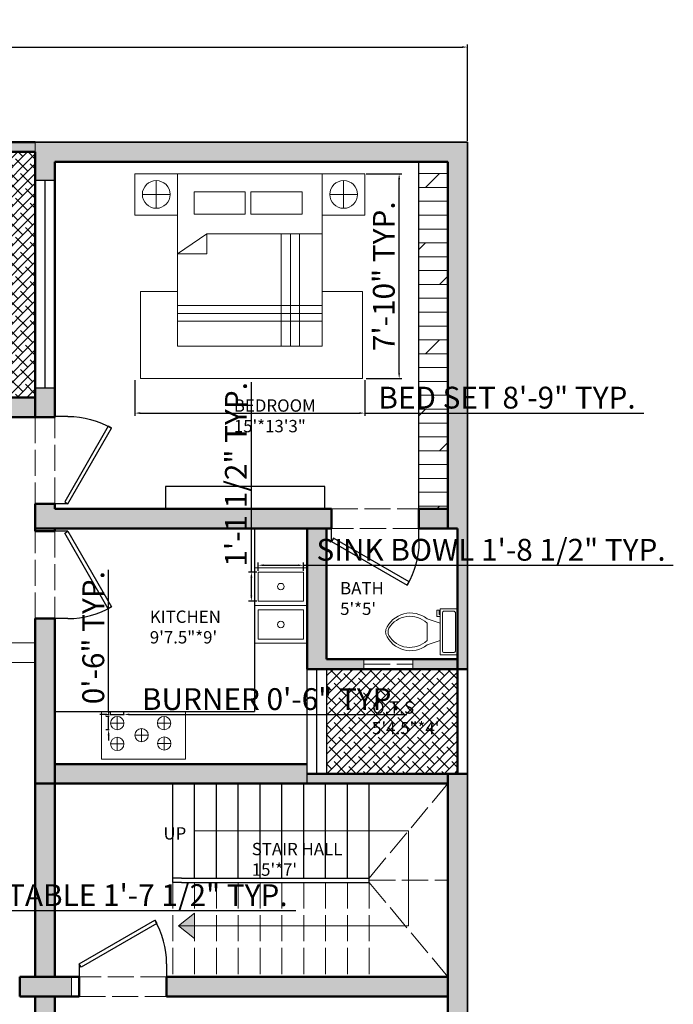
# Model space of a CAD drawing. Units: inches. Extents: x 2101 to 2698, y 3451 to 4160.
# Tile 3 of 3: x 2399 to 2698, y 3709 to 4160. Entities that reach past the tile are written whole.
import ezdxf

# ---------------------------------------------------------------- set-up
doc = ezdxf.new("R2010")
doc.units = ezdxf.units.IN
doc.linetypes.add('ACAD_ISO02W100', pattern=[15, 12, -3])
for name, color, linetype, lineweight in [('A-ANNO-DIMS', 40, 'Continuous', 18), ('A-ANNO-SYMB', 40, 'Continuous', 18), ('A-ANNO-TEXT', 40, 'Continuous', 25), ('A-AREA-IDEN', 40, 'Continuous', 18), ('A-EQPM', 8, 'Continuous', 18), ('A-FLOR-CASE', 132, 'Continuous', 25), ('A-FLOR-CASE-PATT', 132, 'Continuous', 13), ('A-FLOR-FIXT', 9, 'Continuous', 18), ('A-FLOR-PATT', 252, 'Continuous', 13), ('A-FLOR-STRS', 7, 'Continuous', 25), ('A-FLOR-STRS-OVHD', 7, 'ACAD_ISO02W100', 18), ('A-GLAZ-HIDN', 210, 'ACAD_ISO02W100', 18), ('A-WALL-OVHD', 150, 'ACAD_ISO02W100', 18), ('A-WALL-PATT', 150, 'Continuous', 13), ('C-PROP', 7, 'Continuous', 35), ('DOOR', 52, 'Continuous', 25), ('FURNITURE', 132, 'Continuous', 18), ('WALL', 150, 'Continuous', 50), ('WIN', 210, 'Continuous', 25)]:
    doc.layers.add(name, color=color, linetype=linetype, lineweight=lineweight)
doc.styles.get("Standard").update_dxf_attribs({"font": 'arial.ttf'})
doc.dimstyles.new('ISO-25', dxfattribs={"dimtxt": 10, "dimasz": 2.5, "dimexe": 1.25, "dimexo": 0.625, "dimtad": 1, "dimdec": 0, "dimlunit": 4, "dimtxsty": 'Standard', "dimcen": 2.5, "dimadec": 0, "dimazin": 0, "dimtfac": 1, "dimtdec": 0, "dimtmove": 0, "dimatfit": 3, "dimfxl": 1, "dimarcsym": 0})

# ---------------------------------------------------------------- blocks, each defined once
blk = doc.blocks.new('*U2')
for p, q in [((0, 0), (0, -6)), ((40, 0), (40, -6))]:
    blk.add_line(p, q)
blk.add_lwpolyline([(0, 0), (34.64, 20), (35.52, 18.48), (0.87, -1.52)], close=True)
blk.add_arc((0, 0), 40, 0, 30)
blk = doc.blocks.new('*U4')
for p, q in [((9.5, -6), (9.5, -2)), ((-10, -8.5), (-8, -8.5)), ((-10, -9.5), (-10, -8.5)), ((-8, -8.5), (-8, -8)), ((-7, -8), (-7, -9.5)), ((-4, -8), (-6, -14)), ((4, -8), (6, -14)), ((-7, -9.5), (-10, -9.5)), ((4, -14), (-4, -14))]:
    blk.add_line(p, q)
blk.add_lwpolyline([(10.5, -8), (10.5, 0), (-10.5, 0), (-10.5, -8)], close=True)
for points in [[(-9.5, -2), (-9.5, -6)], [(8.5, -1), (-8.5, -1)], [(-8.5, -7), (8.5, -7)]]:
    blk.add_lwpolyline(points)
for centre, radius, start, end in [((-8.62, -1.88), 0.884, 81.8699, 188.1301), ((8.62, -1.88), 0.884, 351.8699, 98.1301), ((-8.62, -6.12), 0.884, 171.8699, 278.1301), ((8.62, -6.12), 0.884, 261.8699, 8.1301), ((3.52, -21.58), 12.17, 141.4691, 247.9714), ((4.2, -21.82), 11.33, 136.3677, 238.9468), ((-3.52, -21.58), 12.17, 292.0284, 38.5307), ((-4.2, -21.82), 11.33, 301.053, 43.6321), ((0, -27.88), 4, 245.7318, 294.2682), ((0, -29), 4, 254.8605, 285.1395)]:
    blk.add_arc(centre, radius, start, end)
blk = doc.blocks.new('*D7')
at = {"layer": 'A-ANNO-DIMS', "color": 0, "lineweight": -2, "transparency": 16777216}
for p, q in [((2147.64, 4104.47), (2147.64, 4148.63)), ((2150.14, 4147.38), (2601.14, 4147.38)), ((2603.64, 4104.47), (2603.64, 4148.63))]:
    blk.add_line(p, q, dxfattribs=at)
at = {"layer": 'A-ANNO-DIMS', "color": 0, "lineweight": 100, "transparency": 16777216}
for points in [[(2150.14, 4147.8), (2150.14, 4146.97), (2147.64, 4147.38)], [(2601.14, 4147.8), (2601.14, 4146.97), (2603.64, 4147.38)]]:
    blk.add_solid(points, dxfattribs=at)
at = {"layer": 'Defpoints', "color": 0, "lineweight": 100, "transparency": 16777216}
for p in [(2603.64, 4147.38), (2147.64, 4103.85), (2603.64, 4103.85)]:
    blk.add_point(p, dxfattribs=at)
at = {"layer": 'A-ANNO-DIMS', "color": 0, "transparency": 16777216, "insert": (2375.64, 4153.12), "char_height": 10, "attachment_point": 5}
blk.add_mtext("38'", dxfattribs=at)
blk = doc.blocks.new('BED-DOUBLE-WITH-NIGHTSTANDS')
for p, q in [((9.75, 84.4), (9.75, 90.75)), ((9.75, 90.75), (9.75, 78.05)), ((95.59, 84.4), (95.59, 90.75)), ((95.59, 90.75), (95.59, 78.05)), ((16.1, 84.4), (3.4, 84.4)), ((9.75, 78.05), (9.75, 84.4)), ((9.75, 84.4), (16.1, 84.4)), ((101.95, 84.4), (89.24, 84.4)), ((95.59, 78.05), (95.59, 84.4)), ((95.59, 84.4), (101.95, 84.4)), ((19.5, 57.15), (32.87, 66.43)), ((85.75, 66.43), (32.87, 66.43)), ((32.87, 66.43), (32.87, 57.15)), ((66.97, 66.43), (66.97, 14.83)), ((71.27, 66.43), (71.27, 14.83)), ((75.39, 66.43), (75.39, 14.83)), ((32.87, 57.15), (19.5, 57.15)), ((19.5, 39.97), (2.47, 39.97)), ((2.47, 39.97), (2.47, 0)), ((104.25, 39.97), (85.75, 39.97)), ((104.25, 0), (104.25, 39.97)), ((85.75, 33.58), (19.5, 33.58)), ((85.75, 29.79), (19.5, 29.79)), ((85.75, 26.32), (19.5, 26.32)), ((2.47, 0), (104.25, 0))]:
    blk.add_line(p, q)
for points in [[(0, 93.85), (19.5, 93.85), (19.5, 74.95), (0, 74.95)], [(19.5, 93.85), (85.75, 93.85), (85.75, 14.83), (19.5, 14.83)], [(85.75, 93.85), (105.24, 93.85), (105.24, 74.95), (85.75, 74.95)], [(27.1, 85.6), (50.52, 85.6), (50.52, 75.29), (27.1, 75.29)], [(53.1, 85.6), (76.53, 85.6), (76.53, 75.29), (53.1, 75.29)]]:
    blk.add_lwpolyline(points, close=True)
for centre in [(9.75, 84.4), (95.59, 84.4)]:
    blk.add_circle(centre, 6.35)
blk = doc.blocks.new('SINK-BOWL')
blk.add_lwpolyline([(0, 13.34), (20.72, 13.34), (20.72, 0), (0, 0)], close=True)
blk.add_circle((10.36, 6.67), 1.48)
blk = doc.blocks.new('COOKTOP-BURNER')
for p, q in [((3.05, 3.05), (3.05, 6.09)), ((3.05, 6.09), (3.05, 0)), ((6.09, 3.05), (0, 3.05)), ((3.05, 0), (3.05, 3.05)), ((3.05, 3.05), (6.09, 3.05))]:
    blk.add_line(p, q)
blk.add_circle((3.05, 3.05), 3.05)
blk = doc.blocks.new('*D15')
at = {"layer": 'A-ANNO-DIMS', "color": 0, "lineweight": -2, "transparency": 16777216}
for p, q in [((2451.32, 3994.82), (2451.32, 3978.41)), ((2556.56, 3994.82), (2556.56, 3978.41)), ((2453.82, 3979.66), (2554.06, 3979.66)), ((2556.56, 3979.66), (2684.48, 3979.66))]:
    blk.add_line(p, q, dxfattribs=at)
at = {"layer": 'A-ANNO-DIMS', "color": 0, "lineweight": 100, "transparency": 16777216}
for points in [[(2453.82, 3980.08), (2453.82, 3979.24), (2451.32, 3979.66)], [(2554.06, 3980.08), (2554.06, 3979.24), (2556.56, 3979.66)]]:
    blk.add_solid(points, dxfattribs=at)
at = {"layer": 'Defpoints', "color": 0, "lineweight": 100, "transparency": 16777216}
for p in [(2451.32, 3995.45), (2556.56, 3995.45), (2556.56, 3979.66)]:
    blk.add_point(p, dxfattribs=at)
at = {"layer": 'A-ANNO-DIMS', "color": 0, "transparency": 16777216, "insert": (2621.77, 3985.45), "char_height": 10, "attachment_point": 5}
blk.add_mtext('BED SET 8\'-9" TYP.', dxfattribs=at)
blk = doc.blocks.new('*D16')
at = {"layer": 'A-ANNO-DIMS', "color": 0, "lineweight": -2, "transparency": 16777216}
for p, q in [((2557.19, 4089.3), (2573.6, 4089.3)), ((2572.35, 3997.95), (2572.35, 4086.8)), ((2557.19, 3995.45), (2573.6, 3995.45))]:
    blk.add_line(p, q, dxfattribs=at)
at = {"layer": 'A-ANNO-DIMS', "color": 0, "lineweight": 100, "transparency": 16777216}
for points in [[(2571.93, 4086.8), (2572.76, 4086.8), (2572.35, 4089.3)], [(2571.93, 3997.95), (2572.76, 3997.95), (2572.35, 3995.45)]]:
    blk.add_solid(points, dxfattribs=at)
at = {"layer": 'Defpoints', "color": 0, "lineweight": 100, "transparency": 16777216}
for p in [(2556.56, 4089.3), (2572.35, 4089.3), (2556.56, 3995.45)]:
    blk.add_point(p, dxfattribs=at)
at = {"layer": 'A-ANNO-DIMS', "color": 0, "transparency": 16777216, "insert": (2566.62, 4042.37), "char_height": 10, "attachment_point": 5, "rotation": 90}
blk.add_mtext('7\'-10" TYP.', dxfattribs=at)
blk = doc.blocks.new('*D17')
at = {"layer": 'A-ANNO-DIMS', "color": 0, "lineweight": -2, "transparency": 16777216}
for p, q in [((2507.76, 3907.45), (2507.76, 3911.18)), ((2510.26, 3909.93), (2525.98, 3909.93)), ((2528.48, 3907.45), (2528.48, 3911.18)), ((2528.48, 3909.93), (2697.94, 3909.93))]:
    blk.add_line(p, q, dxfattribs=at)
at = {"layer": 'A-ANNO-DIMS', "color": 0, "lineweight": 100, "transparency": 16777216}
for points in [[(2510.26, 3910.34), (2510.26, 3909.51), (2507.76, 3909.93)], [(2525.98, 3910.34), (2525.98, 3909.51), (2528.48, 3909.93)]]:
    blk.add_solid(points, dxfattribs=at)
at = {"layer": 'Defpoints', "color": 0, "lineweight": 100, "transparency": 16777216}
for p in [(2528.48, 3909.93), (2507.76, 3906.82), (2528.48, 3906.82)]:
    blk.add_point(p, dxfattribs=at)
at = {"layer": 'A-ANNO-DIMS', "color": 0, "transparency": 16777216, "insert": (2614.46, 3915.73), "char_height": 10, "attachment_point": 5}
blk.add_mtext('SINK BOWL 1\'-8 1/2" TYP.', dxfattribs=at)
blk = doc.blocks.new('*D18')
at = {"layer": 'A-ANNO-DIMS', "color": 0, "lineweight": -2, "transparency": 16777216}
for p, q in [((2504.65, 3906.82), (2504.65, 3993.89)), ((2507.14, 3906.82), (2503.4, 3906.82)), ((2504.65, 3895.98), (2504.65, 3904.32)), ((2507.14, 3893.48), (2503.4, 3893.48))]:
    blk.add_line(p, q, dxfattribs=at)
at = {"layer": 'A-ANNO-DIMS', "color": 0, "lineweight": 100, "transparency": 16777216}
for points in [[(2504.24, 3904.32), (2505.07, 3904.32), (2504.65, 3906.82)], [(2504.24, 3895.98), (2505.07, 3895.98), (2504.65, 3893.48)]]:
    blk.add_solid(points, dxfattribs=at)
at = {"layer": 'Defpoints', "color": 0, "lineweight": 100, "transparency": 16777216}
for p in [(2504.65, 3906.82), (2507.76, 3906.82), (2507.76, 3893.48)]:
    blk.add_point(p, dxfattribs=at)
at = {"layer": 'A-ANNO-DIMS', "color": 0, "transparency": 16777216, "insert": (2498.86, 3951.6), "char_height": 10, "attachment_point": 5, "rotation": 90}
blk.add_mtext('1\'-1 1/2" TYP.', dxfattribs=at)
blk = doc.blocks.new('*D19')
at = {"layer": 'A-ANNO-DIMS', "color": 0, "lineweight": -2, "transparency": 16777216}
for p, q in [((2437.67, 3841.57), (2435.17, 3841.57)), ((2440.17, 3841.28), (2440.17, 3842.82)), ((2440.17, 3841.57), (2446.26, 3841.57)), ((2446.26, 3841.28), (2446.26, 3842.82)), ((2448.76, 3841.57), (2575.9, 3841.57))]:
    blk.add_line(p, q, dxfattribs=at)
at = {"layer": 'A-ANNO-DIMS', "color": 0, "lineweight": 100, "transparency": 16777216}
for points in [[(2437.67, 3841.99), (2437.67, 3841.15), (2440.17, 3841.57)], [(2448.76, 3841.99), (2448.76, 3841.15), (2446.26, 3841.57)]]:
    blk.add_solid(points, dxfattribs=at)
at = {"layer": 'Defpoints', "color": 0, "lineweight": 100, "transparency": 16777216}
for p in [(2440.17, 3840.65), (2446.26, 3841.57), (2446.26, 3840.65)]:
    blk.add_point(p, dxfattribs=at)
at = {"layer": 'A-ANNO-DIMS', "color": 0, "transparency": 16777216, "insert": (2513.58, 3847.3), "char_height": 10, "attachment_point": 5}
blk.add_mtext('BURNER 0\'-6" TYP.', dxfattribs=at)
blk = doc.blocks.new('*D20')
at = {"layer": 'A-ANNO-DIMS', "color": 0, "lineweight": -2, "transparency": 16777216}
for p, q in [((2439.25, 3843.15), (2439.25, 3907.86)), ((2439.54, 3840.65), (2438, 3840.65)), ((2439.25, 3834.56), (2439.25, 3840.65)), ((2439.54, 3834.56), (2438, 3834.56)), ((2439.25, 3832.06), (2439.25, 3829.56))]:
    blk.add_line(p, q, dxfattribs=at)
at = {"layer": 'A-ANNO-DIMS', "color": 0, "lineweight": 100, "transparency": 16777216}
for points in [[(2438.84, 3843.15), (2439.67, 3843.15), (2439.25, 3840.65)], [(2438.84, 3832.06), (2439.67, 3832.06), (2439.25, 3834.56)]]:
    blk.add_solid(points, dxfattribs=at)
at = {"layer": 'Defpoints', "color": 0, "lineweight": 100, "transparency": 16777216}
for p in [(2439.25, 3840.65), (2440.17, 3840.65), (2440.17, 3834.56)]:
    blk.add_point(p, dxfattribs=at)
at = {"layer": 'A-ANNO-DIMS', "color": 0, "transparency": 16777216, "insert": (2433.52, 3876.76), "char_height": 10, "attachment_point": 5, "rotation": 90}
blk.add_mtext('0\'-6" TYP.', dxfattribs=at)
blk = doc.blocks.new('*D25')
at = {"layer": 'A-ANNO-DIMS', "color": 0, "lineweight": -2, "transparency": 16777216}
for p, q in [((2336.34, 3749.33), (2336.34, 3752.92)), ((2338.84, 3751.67), (2353.58, 3751.67)), ((2356.08, 3749.33), (2356.08, 3752.92)), ((2356.08, 3751.67), (2525.08, 3751.67))]:
    blk.add_line(p, q, dxfattribs=at)
at = {"layer": 'A-ANNO-DIMS', "color": 0, "lineweight": 100, "transparency": 16777216}
for points in [[(2338.84, 3752.09), (2338.84, 3751.25), (2336.34, 3751.67)], [(2353.58, 3752.09), (2353.58, 3751.25), (2356.08, 3751.67)]]:
    blk.add_solid(points, dxfattribs=at)
at = {"layer": 'Defpoints', "color": 0, "lineweight": 100, "transparency": 16777216}
for p in [(2356.08, 3751.67), (2336.34, 3748.71), (2356.08, 3748.71)]:
    blk.add_point(p, dxfattribs=at)
at = {"layer": 'A-ANNO-DIMS', "color": 0, "transparency": 16777216, "insert": (2441.83, 3757.46), "char_height": 10, "attachment_point": 5}
blk.add_mtext('END TABLE 1\'-7 1/2" TYP.', dxfattribs=at)

msp = doc.modelspace()

# ---------------------------------------------------------------- hatches: boundary and pattern name
at = {"layer": 'A-ANNO-SYMB'}
h = msp.add_hatch(color=256, dxfattribs=at)
h.dxf.hatch_style = 1
h.paths.add_polyline_path([(2478.64, 3750.44), (2471.33, 3744.68), (2478.64, 3744.68)])
h.paths.add_polyline_path([(2478.64, 3744.68), (2471.33, 3744.68), (2478.64, 3738.91)])
at = {"layer": 'A-FLOR-CASE-PATT'}
h = msp.add_hatch(dxfattribs=at)
h.set_pattern_fill('DOLMIT', color=256)
h.paths.add_polyline_path([(2594.64, 4094.85), (2581.41, 4094.85), (2581.41, 3935.85), (2594.64, 3935.85)])
at = {"layer": 'A-FLOR-PATT'}
h = msp.add_hatch(dxfattribs=at)
h.set_pattern_fill('ANSI38', color=256)
h.paths.add_polyline_path([(2405.64, 4094.85), (2405.64, 4099.35), (2333.64, 4099.35), (2333.64, 4094.85), (2333.64, 4025.85), (2333.64, 3986.85), (2352.22, 3986.85), (2352.22, 3992.85, -0.120537), (2356.74, 4011.31), (2356.7, 4011.33), (2357.58, 4012.85), (2392.22, 3992.85), (2392.22, 3986.85), (2405.64, 3986.85)])
h = msp.add_hatch(dxfattribs=at)
h.set_pattern_fill('ANSI38', color=256)
h.paths.add_polyline_path([(2599.14, 3862.35), (2594.64, 3862.35), (2539.14, 3862.35), (2539.14, 3814.35), (2594.64, 3814.35), (2599.14, 3814.35)])
h.paths.add_polyline_path([(2414.64, 3559.35), (2333.64, 3559.35), (2237.64, 3559.35), (2237.64, 3512.85), (2237.64, 3508.35), (2414.64, 3508.35), (2414.64, 3510.57)])
at = {"layer": 'A-WALL-PATT'}
h = msp.add_hatch(color=256, dxfattribs=at)
h.dxf.hatch_style = 1
h.paths.add_polyline_path([(2333.64, 4094.85), (2333.64, 4099.35), (2324.64, 4099.35), (2324.64, 4094.85), (2324.64, 4083.45), (2333.64, 4083.45)])
h.paths.add_polyline_path([(2405.64, 4103.85), (2156.64, 4103.85), (2156.64, 4099.35), (2405.64, 4099.35)])
h.paths.add_polyline_path([(2156.64, 4099.35), (2147.64, 4099.35), (2147.64, 3721.35), (2156.64, 3721.35)])
h = msp.add_hatch(color=256, dxfattribs=at)
h.dxf.hatch_style = 1
h.paths.add_polyline_path([(2156.64, 4103.85), (2147.64, 4103.85), (2147.64, 4099.35), (2156.64, 4099.35)])
h.paths.add_polyline_path([(2163.74, 4034.85), (2156.64, 4034.85), (2156.64, 4025.85), (2163.74, 4025.85)])
h.paths.add_polyline_path([(2333.64, 3874.35), (2333.64, 3879.64), (2324.64, 3879.64), (2324.64, 3874.35), (2213.91, 3874.35), (2213.91, 3865.35), (2333.64, 3865.35)])
h.paths.add_polyline_path([(2333.64, 3977.85), (2324.64, 3977.85), (2324.64, 3934.78), (2324.64, 3919.64), (2333.64, 3919.64)])
h.paths.add_polyline_path([(2161.58, 3874.35), (2156.64, 3874.35), (2156.64, 3865.35), (2161.58, 3865.35)])
h.paths.add_polyline_path([(2541.41, 3935.85), (2414.64, 3935.85), (2414.64, 3938.14), (2405.64, 3938.14), (2405.64, 3926.85), (2541.41, 3926.85)])
h.paths.add_polyline_path([(2594.64, 3935.85), (2581.41, 3935.85), (2581.41, 3926.85), (2594.64, 3926.85)])
h.paths.add_polyline_path([(2539.14, 3926.85), (2530.14, 3926.85), (2530.14, 3862.35), (2556.24, 3862.35), (2556.24, 3866.85), (2539.14, 3866.85)])
h.paths.add_polyline_path([(2599.14, 3866.85), (2594.64, 3866.85), (2578.65, 3866.85), (2578.65, 3862.35), (2594.64, 3862.35), (2599.14, 3862.35)])
h.paths.add_polyline_path([(2414.64, 3885.48), (2405.64, 3885.48), (2405.64, 3809.85), (2414.64, 3809.85), (2414.64, 3818.85), (2414.64, 3842.85)])
h.paths.add_polyline_path([(2530.14, 3818.85), (2414.64, 3818.85), (2414.64, 3809.85), (2450.64, 3809.85), (2530.14, 3809.85)])
h.paths.add_polyline_path([(2414.64, 3809.85), (2405.64, 3809.85), (2405.64, 3721.35), (2414.64, 3721.35), (2414.64, 3725.85)])
h.paths.add_polyline_path([(2603.64, 3814.35), (2599.14, 3814.35), (2594.64, 3814.35), (2594.64, 3559.35), (2603.64, 3559.35)])
h.paths.add_polyline_path([(2594.64, 3814.35), (2530.14, 3814.35), (2530.14, 3809.85), (2594.64, 3809.85)])
h = msp.add_hatch(color=256, dxfattribs=at)
h.dxf.hatch_style = 1
h.paths.add_polyline_path([(2333.64, 4031.79), (2333.64, 4051.21), (2324.64, 4051.21), (2324.64, 4034.85), (2324.64, 4031.79), (2324.64, 3977.85), (2333.64, 3977.85), (2333.64, 3984.47), (2333.64, 3986.85)])
h.paths.add_polyline_path([(2352.22, 3986.85), (2333.64, 3986.85), (2333.64, 3984.47), (2333.64, 3977.85), (2352.22, 3977.85)])
h.paths.add_polyline_path([(2405.64, 3986.85), (2392.22, 3986.85), (2392.22, 3977.85), (2405.64, 3977.85)])
h.paths.add_polyline_path([(2414.64, 3991.02), (2405.64, 3991.02), (2405.64, 3977.85), (2414.64, 3977.85)], flags=17)
h.paths.add_polyline_path([(2603.64, 4103.85), (2405.64, 4103.85), (2405.64, 4099.35), (2405.64, 4086.33), (2414.64, 4086.33), (2414.64, 4094.85), (2594.64, 4094.85), (2594.64, 3926.85), (2599.14, 3926.85), (2599.14, 3862.35), (2603.64, 3862.35)])
h.paths.add_polyline_path([(2324.64, 4031.79), (2324.64, 4034.85), (2213.11, 4034.85), (2196.16, 4034.85), (2196.16, 4025.85), (2221.14, 4025.85), (2324.64, 4025.85)])
h.paths.add_polyline_path([(2333.64, 4099.35), (2324.64, 4099.35), (2324.64, 4094.85), (2324.64, 4083.45), (2333.64, 4083.45), (2333.64, 4094.85)])
h = msp.add_hatch(color=256, dxfattribs=at)
h.dxf.hatch_style = 1
h.paths.add_polyline_path([(2603.64, 4103.85), (2405.64, 4103.85), (2405.64, 4099.35), (2405.64, 4086.33), (2414.64, 4086.33), (2414.64, 4094.85), (2594.64, 4094.85), (2594.64, 3926.85), (2599.14, 3926.85), (2599.14, 3862.35), (2603.64, 3862.35)])
h = msp.add_hatch(color=256, dxfattribs=at)
h.dxf.hatch_style = 1
h.paths.add_polyline_path([(2324.64, 4031.79), (2324.64, 4034.85), (2213.11, 4034.85), (2196.16, 4034.85), (2196.16, 4025.85), (2221.14, 4025.85), (2324.64, 4025.85)])
h.paths.add_polyline_path([(2163.74, 4034.85), (2156.64, 4034.85), (2156.64, 4025.85), (2163.74, 4025.85)])
h.paths.add_polyline_path([(2333.64, 4094.85), (2333.64, 4099.35), (2324.64, 4099.35), (2324.64, 4094.85), (2324.64, 4083.45), (2333.64, 4083.45)])
h.paths.add_polyline_path([(2333.64, 4051.21), (2324.64, 4051.21), (2324.64, 4034.85), (2324.64, 4031.79), (2324.64, 4025.85), (2324.64, 3977.85), (2333.64, 3977.85), (2333.64, 3984.47), (2333.64, 3986.85), (2333.64, 4031.79)])
h.paths.add_polyline_path([(2333.64, 3977.85), (2324.64, 3977.85), (2324.64, 3934.78), (2324.64, 3919.64), (2333.64, 3919.64)])
h.paths.add_polyline_path([(2352.22, 3986.85), (2333.64, 3986.85), (2333.64, 3984.47), (2333.64, 3977.85), (2352.22, 3977.85)])
h.paths.add_polyline_path([(2405.64, 3986.85), (2392.22, 3986.85), (2392.22, 3977.85), (2405.64, 3977.85)])
h.paths.add_polyline_path([(2414.64, 3991.02), (2405.64, 3991.02), (2405.64, 3977.85), (2414.64, 3977.85)])
h.paths.add_polyline_path([(2161.58, 3874.35), (2156.64, 3874.35), (2156.64, 3865.35), (2161.58, 3865.35)])
h.paths.add_polyline_path([(2333.64, 3879.64), (2324.64, 3879.64), (2324.64, 3874.35), (2213.91, 3874.35), (2213.91, 3865.35), (2333.64, 3865.35)])
h = msp.add_hatch(color=256, dxfattribs=at)
h.dxf.hatch_style = 1
h.paths.add_polyline_path([(2333.64, 4031.79), (2333.64, 4051.21), (2324.64, 4051.21), (2324.64, 4034.85), (2324.64, 4031.79), (2324.64, 3977.85), (2333.64, 3977.85), (2333.64, 3984.47), (2333.64, 3986.85)])
h.paths.add_polyline_path([(2324.64, 4034.85), (2213.11, 4034.85), (2196.16, 4034.85), (2196.16, 4025.85), (2221.14, 4025.85), (2324.64, 4025.85), (2324.64, 4031.79)])
h.paths.add_polyline_path([(2352.22, 3986.85), (2333.64, 3986.85), (2333.64, 3984.47), (2333.64, 3977.85), (2352.22, 3977.85)])
h.paths.add_polyline_path([(2405.64, 3986.85), (2392.22, 3986.85), (2392.22, 3977.85), (2405.64, 3977.85)])
h.paths.add_polyline_path([(2414.64, 3991.02), (2405.64, 3991.02), (2405.64, 3977.85), (2414.64, 3977.85)])
h = msp.add_hatch(color=256, dxfattribs=at)
h.dxf.hatch_style = 1
h.paths.add_polyline_path([(2541.41, 3935.85), (2414.64, 3935.85), (2414.64, 3938.14), (2405.64, 3938.14), (2405.64, 3926.85), (2541.41, 3926.85)], flags=17)
h.paths.add_polyline_path([(2594.64, 3935.85), (2581.41, 3935.85), (2581.41, 3926.85), (2594.64, 3926.85)], flags=17)
h.paths.add_polyline_path([(2414.64, 3885.48), (2405.64, 3885.48), (2405.64, 3809.85), (2414.64, 3809.85), (2414.64, 3818.85)], flags=17)
h.paths.add_polyline_path([(2539.14, 3926.85), (2530.14, 3926.85), (2530.14, 3862.35), (2539.14, 3862.35), (2539.14, 3866.85)], flags=17)
h.paths.add_polyline_path([(2578.65, 3866.85), (2578.65, 3862.35), (2599.14, 3862.35), (2599.14, 3866.85)])
h.paths.add_polyline_path([(2556.24, 3862.35), (2556.24, 3866.85), (2539.14, 3866.85), (2539.14, 3862.35)])
h = msp.add_hatch(color=256, dxfattribs=at)
h.dxf.hatch_style = 1
h.paths.add_polyline_path([(2225.64, 3721.35), (2156.64, 3721.35), (2156.64, 3712.35), (2225.64, 3712.35)])
h.paths.add_polyline_path([(2339.85, 3721.35), (2333.64, 3721.35), (2225.64, 3721.35), (2225.64, 3712.35), (2324.64, 3712.35), (2339.85, 3712.35)])
h.paths.add_polyline_path([(2422.2, 3721.35), (2398.52, 3721.35), (2398.52, 3712.35), (2422.2, 3712.35)])
h.paths.add_polyline_path([(2414.64, 3809.85), (2405.64, 3809.85), (2405.64, 3721.35), (2414.64, 3721.35), (2414.64, 3725.85)])
h.paths.add_polyline_path([(2594.64, 3721.35), (2558.64, 3721.35), (2465.82, 3721.35), (2465.82, 3712.35), (2594.64, 3712.35)])
h.paths.add_polyline_path([(2530.14, 3818.85), (2414.64, 3818.85), (2414.64, 3809.85), (2530.14, 3809.85)])
h.paths.add_polyline_path([(2594.64, 3814.35), (2530.14, 3814.35), (2530.14, 3809.85), (2594.64, 3809.85)])
h = msp.add_hatch(color=256, dxfattribs=at)
h.dxf.hatch_style = 1
h.paths.add_polyline_path([(2594.64, 3721.35), (2558.64, 3721.35), (2465.82, 3721.35), (2465.82, 3712.35), (2594.64, 3712.35)])
h.paths.add_polyline_path([(2530.14, 3818.85), (2414.64, 3818.85), (2414.64, 3809.85), (2450.64, 3809.85), (2530.14, 3809.85)])
h.paths.add_polyline_path([(2594.64, 3814.35), (2530.14, 3814.35), (2530.14, 3809.85), (2594.64, 3809.85)])
h = msp.add_hatch(color=256, dxfattribs=at)
h.dxf.hatch_style = 1
h.paths.add_polyline_path([(2603.64, 3814.35), (2599.14, 3814.35), (2594.64, 3814.35), (2594.64, 3559.35), (2603.64, 3559.35)])
h = msp.add_hatch(color=256, dxfattribs=at)
h.dxf.hatch_style = 1
h.paths.add_polyline_path([(2228.64, 3568.35), (2200.53, 3568.35), (2200.53, 3563.85), (2228.64, 3563.85)])
h.paths.add_polyline_path([(2339.85, 3721.35), (2333.64, 3721.35), (2225.64, 3721.35), (2225.64, 3712.35), (2324.64, 3712.35), (2339.85, 3712.35)])
h.paths.add_polyline_path([(2225.64, 3721.35), (2156.64, 3721.35), (2156.64, 3712.35), (2225.64, 3712.35)])
h.paths.add_polyline_path([(2225.64, 3790), (2216.64, 3790), (2216.64, 3785.85), (2201.25, 3785.85), (2201.25, 3781.35), (2225.64, 3781.35)])
h.paths.add_polyline_path([(2225.64, 3781.35), (2221.14, 3781.35), (2221.14, 3764.71), (2225.64, 3764.71)])
h.paths.add_polyline_path([(2175.48, 3785.85), (2156.64, 3785.85), (2156.64, 3781.35), (2175.48, 3781.35)])
h.paths.add_polyline_path([(2414.64, 3809.85), (2405.64, 3809.85), (2405.64, 3721.35), (2414.64, 3721.35), (2414.64, 3725.85)])
h.paths.add_polyline_path([(2422.2, 3721.35), (2398.52, 3721.35), (2398.52, 3712.35), (2422.2, 3712.35)])
h = msp.add_hatch(color=256, dxfattribs=at)
h.dxf.hatch_style = 1
h.paths.add_polyline_path([(2247.32, 3568.35), (2228.64, 3568.35), (2228.64, 3559.35), (2228.64, 3512.85), (2237.64, 3512.85), (2237.64, 3559.35), (2247.32, 3559.35)])
h.paths.add_polyline_path([(2228.64, 3568.35), (2200.53, 3568.35), (2200.53, 3563.85), (2228.64, 3563.85)])
h.paths.add_polyline_path([(2333.64, 3569.5), (2333.64, 3571.5), (2324.64, 3571.5), (2324.64, 3568.35), (2316.02, 3568.35), (2316.02, 3559.35), (2333.64, 3559.35)])
h.paths.add_polyline_path([(2333.64, 3664.35), (2324.64, 3664.35), (2324.64, 3611.5), (2333.64, 3611.5)])
h.paths.add_polyline_path([(2343.31, 3640.35), (2333.64, 3640.35), (2333.64, 3631.35), (2343.31, 3631.35)])
h.paths.add_polyline_path([(2414.64, 3712.35), (2405.64, 3712.35), (2405.64, 3640.35), (2394.74, 3640.35), (2394.74, 3631.35), (2414.64, 3631.35)])
h = msp.add_hatch(color=256, dxfattribs=at)
h.dxf.hatch_style = 1
h.paths.add_polyline_path([(2333.64, 3571.5), (2324.64, 3571.5), (2324.64, 3568.35), (2316.02, 3568.35), (2316.02, 3559.35), (2333.64, 3559.35)])
h.paths.add_polyline_path([(2237.64, 3559.35), (2247.32, 3559.35), (2247.32, 3568.35), (2228.64, 3568.35), (2228.64, 3559.35), (2228.64, 3512.85), (2237.64, 3512.85)])
h.paths.add_polyline_path([(2421.88, 3510.57), (2414.64, 3510.57), (2414.64, 3503.85), (2421.88, 3503.85)])
h.paths.add_polyline_path([(2603.64, 3510.57), (2596.41, 3510.57), (2596.41, 3503.85), (2603.64, 3503.85)])
h.paths.add_polyline_path([(2333.64, 3664.35), (2324.64, 3664.35), (2324.64, 3611.5), (2333.64, 3611.5)])
h.paths.add_polyline_path([(2414.64, 3712.35), (2405.64, 3712.35), (2405.64, 3640.35), (2394.74, 3640.35), (2394.74, 3631.35), (2414.64, 3631.35)])
h.paths.add_polyline_path([(2343.31, 3640.35), (2333.64, 3640.35), (2333.64, 3631.35), (2343.31, 3631.35)])

# ---------------------------------------------------------------- linework, layer by layer
at = {"layer": 'A-ANNO-SYMB'}
for p, q in [((2478.64, 3788.22), (2576.64, 3788.22)), ((2576.64, 3788.22), (2576.64, 3744.68)), ((2471.33, 3744.68), (2478.64, 3750.44)), ((2478.64, 3750.44), (2478.64, 3738.91)), ((2576.64, 3744.68), (2471.33, 3744.68)), ((2471.33, 3744.68), (2478.64, 3738.91))]:
    msp.add_line(p, q, dxfattribs=at)
at = {"layer": 'A-EQPM'}
msp.add_lwpolyline([(2436.06, 3842.85), (2474.43, 3842.85), (2474.43, 3821.12), (2436.06, 3821.12)], close=True, dxfattribs=at)
at = {"layer": 'A-FLOR-CASE'}
for p, q in [((2581.41, 3935.85), (2581.41, 4094.85)), ((2530.14, 3926.85), (2506.14, 3926.85)), ((2506.14, 3926.85), (2506.14, 3842.85)), ((2414.64, 3818.85), (2414.64, 3842.85)), ((2414.64, 3842.85), (2506.14, 3842.85))]:
    msp.add_line(p, q, dxfattribs=at)
msp.add_lwpolyline([(2465.24, 3935.85), (2538.33, 3935.85), (2538.33, 3946.08), (2465.24, 3946.08)], close=True, dxfattribs=at)
at = {"layer": 'A-FLOR-FIXT'}
msp.add_line((2506.14, 3891.5), (2530.14, 3891.5), dxfattribs=at)
msp.add_lwpolyline([(2506.14, 3908.77), (2530.14, 3908.77), (2530.14, 3874.23), (2506.14, 3874.23)], close=True, dxfattribs=at)
at = {"layer": 'A-FLOR-STRS'}
for p, q in [((2414.64, 3809.85), (2450.64, 3809.85)), ((2468.64, 3764.6), (2468.64, 3809.85)), ((2478.64, 3766.6), (2478.64, 3809.85)), ((2488.64, 3766.6), (2488.64, 3809.85)), ((2498.64, 3766.6), (2498.64, 3809.85)), ((2508.64, 3766.6), (2508.64, 3809.85)), ((2518.64, 3766.6), (2518.64, 3809.85)), ((2528.64, 3766.6), (2528.64, 3809.85)), ((2538.64, 3766.6), (2538.64, 3809.85)), ((2548.64, 3766.6), (2548.64, 3809.85)), ((2558.64, 3764.6), (2558.64, 3809.85)), ((2472.58, 3766.6), (2468.64, 3766.6)), ((2472.58, 3764.6), (2468.64, 3764.6)), ((2472.58, 3766.6), (2558.64, 3766.6)), ((2472.58, 3764.6), (2558.64, 3764.6)), ((2594.64, 3721.35), (2558.64, 3721.35))]:
    msp.add_line(p, q, dxfattribs=at)
at = {"layer": 'A-FLOR-STRS-OVHD'}
for p, q in [((2558.64, 3766.6), (2594.64, 3809.85)), ((2468.64, 3764.6), (2468.64, 3721.35)), ((2478.64, 3764.6), (2478.64, 3721.35)), ((2488.64, 3764.6), (2488.64, 3721.35)), ((2498.64, 3764.6), (2498.64, 3721.35)), ((2508.64, 3764.6), (2508.64, 3721.35)), ((2518.64, 3764.6), (2518.64, 3721.35)), ((2528.64, 3764.6), (2528.64, 3721.35)), ((2538.64, 3764.6), (2538.64, 3721.35)), ((2548.64, 3764.6), (2548.64, 3721.35)), ((2558.64, 3765.61), (2594.64, 3765.61)), ((2558.64, 3764.6), (2558.64, 3721.35)), ((2558.64, 3764.6), (2594.64, 3721.35))]:
    msp.add_line(p, q, dxfattribs=at)
at = {"layer": 'A-GLAZ-HIDN'}
msp.add_line((2556.24, 3864.6), (2578.65, 3864.6), dxfattribs=at)
msp.add_lwpolyline([(2556.24, 3866.85), (2578.65, 3866.85), (2578.65, 3862.35), (2556.24, 3862.35)], close=True, dxfattribs=at)
at = {"layer": 'A-WALL-OVHD'}
msp.add_line((2422.2, 3721.35), (2422.2, 3712.35), dxfattribs=at)
msp.add_lwpolyline([(2147.64, 4099.35), (2147.64, 4103.85), (2405.64, 4103.85), (2405.64, 4099.35), (2156.64, 4099.35)], dxfattribs=at)
for points in [[(2405.64, 3938.14), (2414.64, 3938.14), (2414.64, 3977.85), (2405.64, 3977.85)], [(2541.41, 3935.85), (2581.41, 3935.85), (2581.41, 3926.85), (2541.41, 3926.85)], [(2405.64, 3925.48), (2414.64, 3925.48), (2414.64, 3885.48), (2405.64, 3885.48)], [(2333.64, 3865.35), (2405.64, 3865.35), (2405.64, 3874.35), (2333.64, 3874.35)], [(2425.82, 3712.35), (2465.82, 3712.35), (2465.82, 3721.35), (2425.82, 3721.35)]]:
    msp.add_lwpolyline(points, close=True, dxfattribs=at)
at = {"layer": 'C-PROP'}
for p, q in [((2147.64, 4103.85), (2603.64, 4103.85)), ((2603.64, 4103.85), (2603.64, 3503.85))]:
    msp.add_line(p, q, dxfattribs=at)
at = {"layer": 'WALL'}
for p, q in [((2147.64, 4103.85), (2405.64, 4103.85)), ((2156.64, 4099.35), (2405.64, 4099.35)), ((2333.64, 4099.35), (2405.64, 4099.35)), ((2405.64, 4099.35), (2405.64, 3986.85)), ((2405.64, 4094.85), (2405.64, 3977.85)), ((2414.64, 4094.85), (2414.64, 3977.85)), ((2414.64, 4094.85), (2594.64, 4094.85)), ((2414.64, 4094.85), (2414.64, 3977.85)), ((2594.64, 4094.85), (2594.64, 3926.85)), ((2405.64, 3986.85), (2392.22, 3986.85)), ((2405.64, 3977.85), (2392.22, 3977.85)), ((2405.64, 3938.14), (2405.64, 3926.85)), ((2414.64, 3938.14), (2414.64, 3935.85)), ((2414.64, 3935.85), (2541.41, 3935.85)), ((2581.41, 3935.85), (2594.64, 3935.85)), ((2405.64, 3926.85), (2541.41, 3926.85)), ((2405.64, 3926.85), (2405.64, 3925.48)), ((2530.14, 3926.85), (2414.64, 3926.85)), ((2414.64, 3926.85), (2414.64, 3925.48)), ((2530.14, 3862.35), (2530.14, 3926.85)), ((2539.14, 3866.85), (2539.14, 3926.85)), ((2581.41, 3926.85), (2594.64, 3926.85)), ((2594.64, 3926.85), (2599.14, 3926.85)), ((2599.14, 3926.85), (2599.14, 3814.35)), ((2414.64, 3885.48), (2405.64, 3885.48)), ((2405.64, 3885.48), (2405.64, 3809.85)), ((2414.64, 3885.48), (2414.64, 3818.85)), ((2594.64, 3866.85), (2539.14, 3866.85)), ((2594.64, 3866.85), (2599.14, 3866.85)), ((2594.64, 3862.35), (2530.14, 3862.35)), ((2594.64, 3862.35), (2599.14, 3862.35)), ((2599.14, 3862.35), (2603.64, 3862.35)), ((2405.64, 3721.35), (2405.64, 3818.85)), ((2414.64, 3818.85), (2530.14, 3818.85)), ((2414.64, 3725.85), (2414.64, 3818.85)), ((2594.64, 3814.35), (2530.14, 3814.35)), ((2594.64, 3814.35), (2594.64, 3559.35)), ((2594.64, 3814.35), (2599.14, 3814.35)), ((2599.14, 3814.35), (2603.64, 3814.35)), ((2530.14, 3809.85), (2405.64, 3809.85)), ((2594.64, 3809.85), (2530.14, 3809.85)), ((2594.64, 3809.85), (2594.64, 3725.85)), ((2414.64, 3725.85), (2414.64, 3721.35)), ((2398.52, 3721.35), (2398.52, 3712.35)), ((2398.52, 3721.35), (2425.82, 3721.35)), ((2465.82, 3721.35), (2594.64, 3721.35)), ((2398.52, 3712.35), (2425.82, 3712.35)), ((2405.64, 3640.35), (2405.64, 3712.35)), ((2414.64, 3631.35), (2414.64, 3712.35)), ((2465.82, 3712.35), (2594.64, 3712.35))]:
    msp.add_line(p, q, dxfattribs=at)
for points in [[(2405.64, 3977.85), (2414.64, 3977.85)], [(2414.64, 3938.14), (2405.64, 3938.14)], [(2541.41, 3935.85), (2541.41, 3926.85)], [(2581.41, 3926.85), (2581.41, 3935.85)], [(2414.64, 3925.48), (2405.64, 3925.48)], [(2405.64, 3885.48), (2414.64, 3885.48)], [(2425.82, 3712.35), (2425.82, 3721.35)], [(2465.82, 3721.35), (2465.82, 3712.35)]]:
    msp.add_lwpolyline(points, dxfattribs=at)
at = {"layer": 'WIN'}
for p, q in [((2410.14, 3991.02), (2410.14, 4086.33)), ((2530.14, 3809.85), (2530.14, 3862.35)), ((2534.64, 3814.35), (2534.64, 3862.35)), ((2539.14, 3862.35), (2539.14, 3814.35)), ((2530.14, 3814.35), (2539.14, 3814.35))]:
    msp.add_line(p, q, dxfattribs=at)
msp.add_lwpolyline([(2405.64, 4086.33), (2414.64, 4086.33), (2414.64, 3991.02), (2405.64, 3991.02)], close=True, dxfattribs=at)

# ---------------------------------------------------------------- block references
at = {"layer": 'A-EQPM'}
for p in [(2440.17, 3834.56), (2461.59, 3834.56), (2440.17, 3824.99), (2451.3, 3829.02), (2461.7, 3825.2)]:
    msp.add_blockref('COOKTOP-BURNER', p, dxfattribs=at)
at = {"layer": 'A-FLOR-FIXT'}
for p in [(2507.76, 3893.48), (2507.76, 3876.14)]:
    msp.add_blockref('SINK-BOWL', p, dxfattribs=at)
at = {"layer": 'A-FLOR-FIXT', "rotation": 270}
msp.add_blockref('*U4', (2599.14, 3879.41), dxfattribs=at)
at = {"layer": 'DOOR', "xscale": -1}
for p, rotation in [((2420.64, 3938.14), 270), ((2541.41, 3920.85), 180)]:
    msp.add_blockref('*U2', p, dxfattribs=dict(at, rotation=rotation))
at = {"layer": 'DOOR', "rotation": 270}
msp.add_blockref('*U2', (2420.64, 3925.48), dxfattribs=at)
at = {"layer": 'DOOR'}
msp.add_blockref('*U2', (2425.82, 3727.35), dxfattribs=at)
at = {"layer": 'FURNITURE'}
msp.add_blockref('BED-DOUBLE-WITH-NIGHTSTANDS', (2451.32, 3995.45), dxfattribs=at)

# ---------------------------------------------------------------- texts
at = {"layer": 'A-ANNO-TEXT', "insert": (2464.37, 3789.91), "char_height": 5.657, "attachment_point": 1}
msp.add_mtext_dynamic_manual_height_columns('UP', width=91.5864, gutter_width=28.28, heights=[0], dxfattribs=at)
at = {"layer": 'A-AREA-IDEN', "char_height": 5.657, "attachment_point": 1}
for s, insert in [('BEDROOM\\P15\'*13\'3"', (2496.62, 3985.95)), ("BATH\\P5'*5'", (2545.31, 3902.25)), ('KITCHEN\\P9\'7.5"*9\'', (2458.14, 3889.18)), ('O.T.S \\P5\'4.5"*4\'', (2559.97, 3847.58)), ("STAIR HALL\\P15'*7'", (2504.83, 3782.72))]:
    msp.add_mtext_dynamic_manual_height_columns(s, width=91.5864, gutter_width=28.28, heights=[0], dxfattribs=dict(at, insert=insert))

# ---------------------------------------------------------------- dimensions: what is measured, and where the dimension line sits
at = {"layer": 'A-ANNO-DIMS'}
dim = msp.add_linear_dim(base=(2603.64, 4147.38), p1=(2147.64, 4103.85), p2=(2603.64, 4103.85), dimstyle='ISO-25', override={"dimclrd": 0, "dimclre": 0, "dimclrt": 0}, dxfattribs=at)
dim.commit()
dim.dimension.update_dxf_attribs({"geometry": '*D7', "text_midpoint": (2375.64, 4153.12)})
for base, p1, p2, picture, middle in [((2572.348, 4089.2961), (2556.5617, 3995.4453), (2556.5617, 4089.2961), '*D16', (2566.6173, 4042.3707)), ((2504.65, 3906.82), (2507.76, 3893.48), (2507.76, 3906.82), '*D18', (2498.86, 3951.6)), ((2439.25, 3840.65), (2440.17, 3834.56), (2440.17, 3840.65), '*D20', (2433.52, 3876.76))]:
    dim = msp.add_linear_dim(base=base, p1=p1, p2=p2, angle=90, text='<> TYP.', dimstyle='ISO-25', override={"dimdec": 1, "dimlfac": 1, "dimrnd": 0, "dimzin": 1, "dimdsep": 46, "dimlunit": 4, "dimfrac": 2}, dxfattribs=at)
    dim.commit()
    dim.dimension.update_dxf_attribs({"geometry": picture, "text_midpoint": middle})
for base, p1, p2, text, picture, middle in [((2556.56, 3979.66), (2451.32, 3995.45), (2556.56, 3995.45), 'BED SET <> TYP.', '*D15', (2621.77, 3985.45)), ((2528.48, 3909.93), (2507.76, 3906.82), (2528.48, 3906.82), 'SINK BOWL <> TYP.', '*D17', (2614.46, 3915.73)), ((2446.26, 3841.57), (2440.17, 3840.65), (2446.26, 3840.65), 'BURNER <> TYP.', '*D19', (2513.58, 3847.3)), ((2356.08, 3751.67), (2336.34, 3748.71), (2356.08, 3748.71), 'END TABLE <> TYP.', '*D25', (2441.83, 3757.46))]:
    dim = msp.add_linear_dim(base=base, p1=p1, p2=p2, text=text, dimstyle='ISO-25', override={"dimdec": 1, "dimlfac": 1, "dimrnd": 0, "dimzin": 1, "dimdsep": 46, "dimlunit": 4, "dimfrac": 2}, dxfattribs=at)
    dim.commit()
    dim.dimension.update_dxf_attribs({"geometry": picture, "text_midpoint": middle})

doc.saveas('drawing.dxf')
